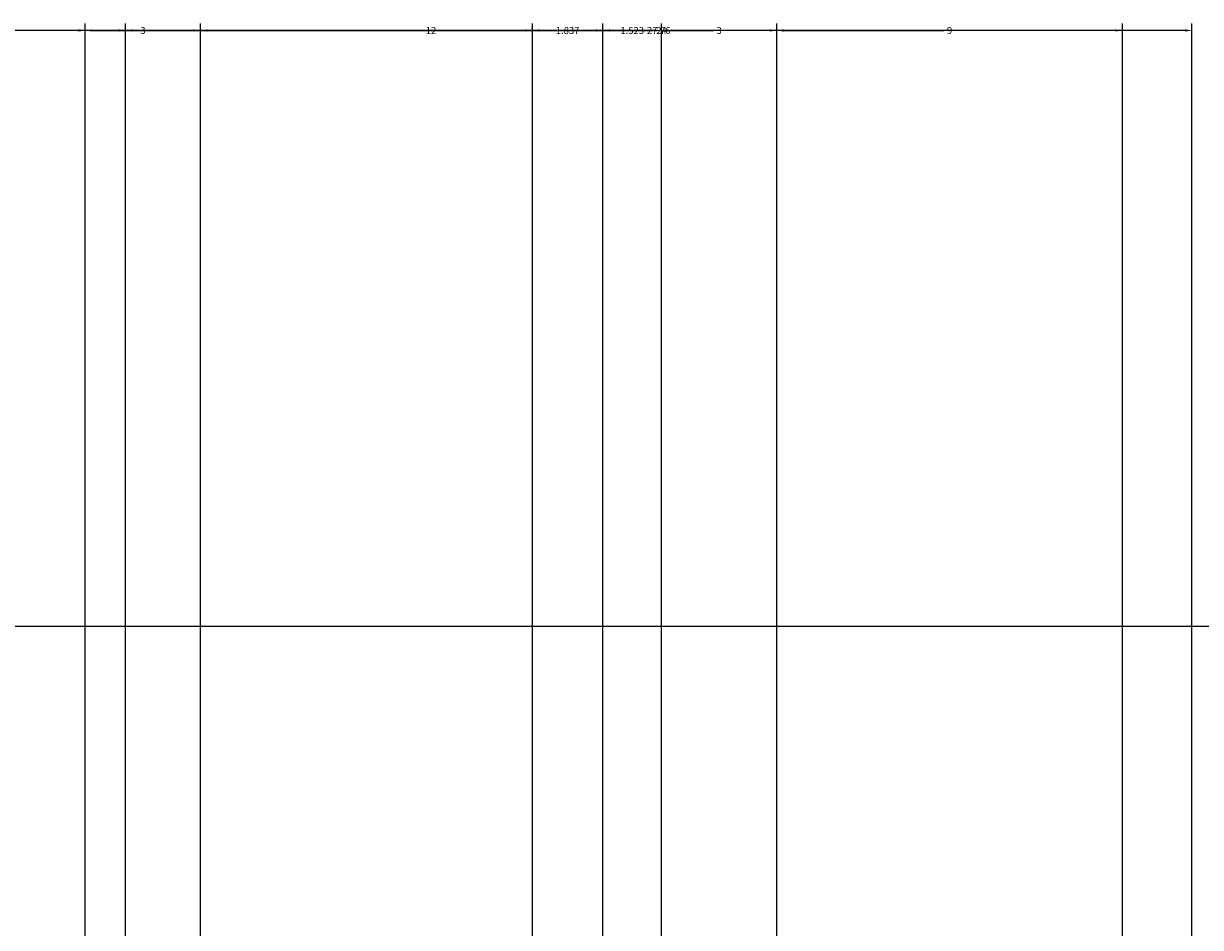
# Model space of a CAD drawing. Units: inches. Extents: x -6 to 289, y -8 to 323.
# Tile 106 of 107: x 243 to 273, y 299 to 323. Entities that reach past the tile are written whole.
import ezdxf

# ---------------------------------------------------------------- set-up
doc = ezdxf.new("R2010")
doc.units = ezdxf.units.IN
doc.header["$MEASUREMENT"] = 0
doc.layers.add('A-ANNO-DIMS', color=2, linetype='Continuous', lineweight=18)
doc.styles.get("Standard").update_dxf_attribs({"font": 'arial.ttf'})
doc.dimstyles.get("Standard").update_dxf_attribs({"dimtxt": 0.18, "dimasz": 0.18, "dimexe": 0.18, "dimexo": 0.0625, "dimgap": 0.09, "dimtad": 0, "dimtih": 1, "dimtoh": 1, "dimdec": 4, "dimzin": 0, "dimdsep": 46, "dimtxsty": 'Standard', "dimcen": 0.09, "dimadec": 0, "dimazin": 0, "dimtfac": 1, "dimtdec": 4, "dimtofl": 0, "dimtmove": 0, "dimatfit": 3, "dimfxl": 1, "dimtolj": 1, "dimtzin": 0, "dimarcsym": 0})

# ---------------------------------------------------------------- blocks, each defined once
blk = doc.blocks.new('*D14')
at = {"layer": 'A-ANNO-DIMS', "color": 0, "lineweight": -2, "transparency": 16777216}
for p, q in [((236.292, 226.951), (236.292, 322.969)), ((247.164, 162.411), (247.164, 322.969)), ((236.472, 322.789), (241.274, 322.789)), ((246.984, 322.789), (242.182, 322.789))]:
    blk.add_line(p, q, dxfattribs=at)
at = {"layer": 'A-ANNO-DIMS', "color": 0, "transparency": 16777216}
for points in [[(236.472, 322.819), (236.472, 322.759), (236.292, 322.789)], [(246.984, 322.819), (246.984, 322.759), (247.164, 322.789)]]:
    blk.add_solid(points, dxfattribs=at)
at = {"layer": 'Defpoints', "color": 0, "transparency": 16777216}
for p in [(247.164, 322.789), (236.292, 226.889), (247.164, 162.348)]:
    blk.add_point(p, dxfattribs=at)
at = {"layer": 'A-ANNO-DIMS', "color": 0, "transparency": 16777216, "insert": (241.728, 322.789), "char_height": 0.18, "attachment_point": 5}
blk.add_mtext('\\A1;10.872', dxfattribs=at)
blk = doc.blocks.new('*D15')
at = {"layer": 'A-ANNO-DIMS', "color": 0, "lineweight": -2, "transparency": 16777216}
for p, q in [((247.164, 162.411), (247.164, 322.969)), ((271.164, 7.351), (271.164, 322.969)), ((247.344, 322.789), (258.944, 322.789)), ((270.984, 322.789), (259.384, 322.789))]:
    blk.add_line(p, q, dxfattribs=at)
at = {"layer": 'A-ANNO-DIMS', "color": 0, "transparency": 16777216}
for points in [[(247.344, 322.819), (247.344, 322.759), (247.164, 322.789)], [(270.984, 322.819), (270.984, 322.759), (271.164, 322.789)]]:
    blk.add_solid(points, dxfattribs=at)
at = {"layer": 'Defpoints', "color": 0, "transparency": 16777216}
for p in [(271.164, 322.789), (247.164, 162.348), (271.164, 7.289)]:
    blk.add_point(p, dxfattribs=at)
at = {"layer": 'A-ANNO-DIMS', "color": 0, "transparency": 16777216, "insert": (259.164, 322.789), "char_height": 0.18, "attachment_point": 5}
blk.add_mtext('\\A1;24', dxfattribs=at)
blk = doc.blocks.new('*D27')
at = {"layer": 'A-ANNO-DIMS', "color": 0, "lineweight": -2, "transparency": 16777216}
for p, q in [((19.226, 307.289), (288.653, 307.289)), ((288.473, 307.109), (288.473, 277.471)), ((288.473, 247.469), (288.473, 277.107)), ((247.226, 247.289), (288.653, 247.289))]:
    blk.add_line(p, q, dxfattribs=at)
at = {"layer": 'A-ANNO-DIMS', "color": 0, "transparency": 16777216}
for points in [[(288.443, 307.109), (288.503, 307.109), (288.473, 307.289)], [(288.443, 247.469), (288.503, 247.469), (288.473, 247.289)]]:
    blk.add_solid(points, dxfattribs=at)
at = {"layer": 'Defpoints', "color": 0, "transparency": 16777216}
for p in [(19.164, 307.289), (288.473, 307.289), (247.164, 247.289)]:
    blk.add_point(p, dxfattribs=at)
at = {"layer": 'A-ANNO-DIMS', "color": 0, "transparency": 16777216, "insert": (288.473, 277.289), "char_height": 0.18, "attachment_point": 5}
blk.add_mtext('\\A1;60', dxfattribs=at)
blk = doc.blocks.new('*D81')
at = {"layer": 'A-ANNO-DIMS', "color": 0, "lineweight": -2, "transparency": 16777216}
for p, q in [((230.292, 68.842), (230.292, 322.969)), ((245.215, 66.286), (245.215, 322.969)), ((230.472, 322.789), (237.298, 322.789)), ((245.035, 322.789), (238.208, 322.789))]:
    blk.add_line(p, q, dxfattribs=at)
at = {"layer": 'A-ANNO-DIMS', "color": 0, "transparency": 16777216}
for points in [[(230.472, 322.819), (230.472, 322.759), (230.292, 322.789)], [(245.035, 322.819), (245.035, 322.759), (245.215, 322.789)]]:
    blk.add_solid(points, dxfattribs=at)
at = {"layer": 'Defpoints', "color": 0, "transparency": 16777216}
for p in [(245.215, 322.789), (230.292, 68.779), (245.215, 66.224)]:
    blk.add_point(p, dxfattribs=at)
at = {"layer": 'A-ANNO-DIMS', "color": 0, "transparency": 16777216, "insert": (237.753, 322.789), "char_height": 0.18, "attachment_point": 5}
blk.add_mtext('\\A1;14.923', dxfattribs=at)
blk = doc.blocks.new('*D82')
at = {"layer": 'A-ANNO-DIMS', "color": 0, "lineweight": -2, "transparency": 16777216}
for p, q in [((245.215, 66.286), (245.215, 322.969)), ((272.973, 66.286), (272.973, 322.969)), ((245.395, 322.789), (258.699, 322.789)), ((272.793, 322.789), (259.489, 322.789))]:
    blk.add_line(p, q, dxfattribs=at)
at = {"layer": 'A-ANNO-DIMS', "color": 0, "transparency": 16777216}
for points in [[(245.395, 322.819), (245.395, 322.759), (245.215, 322.789)], [(272.793, 322.819), (272.793, 322.759), (272.973, 322.789)]]:
    blk.add_solid(points, dxfattribs=at)
at = {"layer": 'Defpoints', "color": 0, "transparency": 16777216}
for p in [(272.973, 322.789), (245.215, 66.224), (272.973, 66.224)]:
    blk.add_point(p, dxfattribs=at)
at = {"layer": 'A-ANNO-DIMS', "color": 0, "transparency": 16777216, "insert": (259.094, 322.789), "char_height": 0.18, "attachment_point": 5}
blk.add_mtext('\\A1;27.76', dxfattribs=at)
blk = doc.blocks.new('*D98')
at = {"layer": 'A-ANNO-DIMS', "color": 0, "lineweight": -2, "transparency": 16777216}
for p, q in [((202.741, 159.411), (202.741, 322.969)), ((244.164, 159.411), (244.164, 322.969)), ((202.921, 322.789), (223.056, 322.789)), ((243.984, 322.789), (223.849, 322.789))]:
    blk.add_line(p, q, dxfattribs=at)
at = {"layer": 'A-ANNO-DIMS', "color": 0, "transparency": 16777216}
for points in [[(202.921, 322.819), (202.921, 322.759), (202.741, 322.789)], [(243.984, 322.819), (243.984, 322.759), (244.164, 322.789)]]:
    blk.add_solid(points, dxfattribs=at)
at = {"layer": 'Defpoints', "color": 0, "transparency": 16777216}
for p in [(244.164, 322.789), (202.741, 159.348), (244.164, 159.348)]:
    blk.add_point(p, dxfattribs=at)
at = {"layer": 'A-ANNO-DIMS', "color": 0, "transparency": 16777216, "insert": (223.452, 322.789), "char_height": 0.18, "attachment_point": 5}
blk.add_mtext('\\A1;41.42', dxfattribs=at)
blk = doc.blocks.new('*D99')
at = {"layer": 'A-ANNO-DIMS', "color": 0, "lineweight": -2, "transparency": 16777216}
for p, q in [((244.164, 159.411), (244.164, 322.969)), ((247.164, 162.411), (247.164, 322.969)), ((244.344, 322.789), (245.515, 322.789)), ((246.984, 322.789), (245.813, 322.789))]:
    blk.add_line(p, q, dxfattribs=at)
at = {"layer": 'A-ANNO-DIMS', "color": 0, "transparency": 16777216}
for points in [[(244.344, 322.819), (244.344, 322.759), (244.164, 322.789)], [(246.984, 322.819), (246.984, 322.759), (247.164, 322.789)]]:
    blk.add_solid(points, dxfattribs=at)
at = {"layer": 'Defpoints', "color": 0, "transparency": 16777216}
for p in [(247.164, 322.789), (247.164, 162.348), (244.164, 159.348)]:
    blk.add_point(p, dxfattribs=at)
at = {"layer": 'A-ANNO-DIMS', "color": 0, "transparency": 16777216, "insert": (245.664, 322.789), "char_height": 0.18, "attachment_point": 5}
blk.add_mtext('\\A1;3', dxfattribs=at)
blk = doc.blocks.new('*D100')
at = {"layer": 'A-ANNO-DIMS', "color": 0, "lineweight": -2, "transparency": 16777216}
for p, q in [((247.164, 162.411), (247.164, 322.969)), ((259.164, 139.351), (259.164, 322.969)), ((247.344, 322.789), (252.954, 322.789)), ((258.984, 322.789), (253.373, 322.789))]:
    blk.add_line(p, q, dxfattribs=at)
at = {"layer": 'A-ANNO-DIMS', "color": 0, "transparency": 16777216}
for points in [[(247.344, 322.819), (247.344, 322.759), (247.164, 322.789)], [(258.984, 322.819), (258.984, 322.759), (259.164, 322.789)]]:
    blk.add_solid(points, dxfattribs=at)
at = {"layer": 'Defpoints', "color": 0, "transparency": 16777216}
for p in [(259.164, 322.789), (247.164, 162.348), (259.164, 139.289)]:
    blk.add_point(p, dxfattribs=at)
at = {"layer": 'A-ANNO-DIMS', "color": 0, "transparency": 16777216, "insert": (253.164, 322.789), "char_height": 0.18, "attachment_point": 5}
blk.add_mtext('\\A1;12', dxfattribs=at)
blk = doc.blocks.new('*D108')
at = {"layer": 'A-ANNO-DIMS', "color": 0, "lineweight": -2, "transparency": 16777216}
for p, q in [((186.984, 291.541), (186.984, 322.969)), ((255.804, 291.541), (255.804, 322.969)), ((187.164, 322.789), (221, 322.789)), ((255.624, 322.789), (221.787, 322.789))]:
    blk.add_line(p, q, dxfattribs=at)
at = {"layer": 'A-ANNO-DIMS', "color": 0, "transparency": 16777216}
for points in [[(187.164, 322.819), (187.164, 322.759), (186.984, 322.789)], [(255.624, 322.819), (255.624, 322.759), (255.804, 322.789)]]:
    blk.add_solid(points, dxfattribs=at)
at = {"layer": 'Defpoints', "color": 0, "transparency": 16777216}
for p in [(255.804, 322.789), (186.984, 291.478), (255.804, 291.478)]:
    blk.add_point(p, dxfattribs=at)
at = {"layer": 'A-ANNO-DIMS', "color": 0, "transparency": 16777216, "insert": (221.394, 322.789), "char_height": 0.18, "attachment_point": 5}
blk.add_mtext('\\A1;68.82', dxfattribs=at)
blk = doc.blocks.new('*D109')
at = {"layer": 'A-ANNO-DIMS', "color": 0, "lineweight": -2, "transparency": 16777216}
for p, q in [((255.804, 291.541), (255.804, 322.969)), ((257.641, 293.728), (257.641, 322.969)), ((255.984, 322.789), (256.337, 322.789)), ((257.461, 322.789), (257.107, 322.789))]:
    blk.add_line(p, q, dxfattribs=at)
at = {"layer": 'A-ANNO-DIMS', "color": 0, "transparency": 16777216}
for points in [[(255.984, 322.819), (255.984, 322.759), (255.804, 322.789)], [(257.461, 322.819), (257.461, 322.759), (257.641, 322.789)]]:
    blk.add_solid(points, dxfattribs=at)
at = {"layer": 'Defpoints', "color": 0, "transparency": 16777216}
for p in [(257.641, 322.789), (257.641, 293.666), (255.804, 291.478)]:
    blk.add_point(p, dxfattribs=at)
at = {"layer": 'A-ANNO-DIMS', "color": 0, "transparency": 16777216, "insert": (256.722, 322.789), "char_height": 0.18, "attachment_point": 5}
blk.add_mtext('\\A1;1.837', dxfattribs=at)
blk = doc.blocks.new('*D110')
at = {"layer": 'A-ANNO-DIMS', "color": 0, "lineweight": -2, "transparency": 16777216}
for p, q in [((257.641, 293.728), (257.641, 322.969)), ((259.164, 277.105), (259.164, 322.969)), ((257.821, 322.789), (258.017, 322.789)), ((258.984, 322.789), (258.787, 322.789))]:
    blk.add_line(p, q, dxfattribs=at)
at = {"layer": 'A-ANNO-DIMS', "color": 0, "transparency": 16777216}
for points in [[(257.821, 322.819), (257.821, 322.759), (257.641, 322.789)], [(258.984, 322.819), (258.984, 322.759), (259.164, 322.789)]]:
    blk.add_solid(points, dxfattribs=at)
at = {"layer": 'Defpoints', "color": 0, "transparency": 16777216}
for p in [(259.164, 322.789), (257.641, 293.666), (259.164, 277.043)]:
    blk.add_point(p, dxfattribs=at)
at = {"layer": 'A-ANNO-DIMS', "color": 0, "transparency": 16777216, "insert": (258.402, 322.789), "char_height": 0.18, "attachment_point": 5}
blk.add_mtext('\\A1;1.523', dxfattribs=at)
blk = doc.blocks.new('*D111')
at = {"layer": 'A-ANNO-DIMS', "color": 0, "lineweight": -2, "transparency": 16777216}
for p, q in [((259.164, 277.105), (259.164, 322.969)), ((262.164, 280.105), (262.164, 322.969)), ((259.344, 322.789), (260.515, 322.789)), ((261.984, 322.789), (260.813, 322.789))]:
    blk.add_line(p, q, dxfattribs=at)
at = {"layer": 'A-ANNO-DIMS', "color": 0, "transparency": 16777216}
for points in [[(259.344, 322.819), (259.344, 322.759), (259.164, 322.789)], [(261.984, 322.819), (261.984, 322.759), (262.164, 322.789)]]:
    blk.add_solid(points, dxfattribs=at)
at = {"layer": 'Defpoints', "color": 0, "transparency": 16777216}
for p in [(262.164, 322.789), (262.164, 280.043), (259.164, 277.043)]:
    blk.add_point(p, dxfattribs=at)
at = {"layer": 'A-ANNO-DIMS', "color": 0, "transparency": 16777216, "insert": (260.664, 322.789), "char_height": 0.18, "attachment_point": 5}
blk.add_mtext('\\A1;3', dxfattribs=at)
blk = doc.blocks.new('*D112')
at = {"layer": 'A-ANNO-DIMS', "color": 0, "lineweight": -2, "transparency": 16777216}
for p, q in [((262.164, 280.105), (262.164, 322.969)), ((271.164, 259.351), (271.164, 322.969)), ((262.344, 322.789), (266.515, 322.789)), ((270.984, 322.789), (266.813, 322.789))]:
    blk.add_line(p, q, dxfattribs=at)
at = {"layer": 'A-ANNO-DIMS', "color": 0, "transparency": 16777216}
for points in [[(262.344, 322.819), (262.344, 322.759), (262.164, 322.789)], [(270.984, 322.819), (270.984, 322.759), (271.164, 322.789)]]:
    blk.add_solid(points, dxfattribs=at)
at = {"layer": 'Defpoints', "color": 0, "transparency": 16777216}
for p in [(271.164, 322.789), (262.164, 280.043), (271.164, 259.289)]:
    blk.add_point(p, dxfattribs=at)
at = {"layer": 'A-ANNO-DIMS', "color": 0, "transparency": 16777216, "insert": (266.664, 322.789), "char_height": 0.18, "attachment_point": 5}
blk.add_mtext('\\A1;9', dxfattribs=at)
blk = doc.blocks.new('*D118')
at = {"layer": 'A-ANNO-DIMS', "color": 0, "lineweight": -2, "transparency": 16777216}
for p, q in [((118.226, 307.289), (288.653, 307.289)), ((288.473, 307.109), (288.473, 300.659)), ((288.473, 293.846), (288.473, 300.295)), ((257.703, 293.666), (288.653, 293.666))]:
    blk.add_line(p, q, dxfattribs=at)
at = {"layer": 'A-ANNO-DIMS', "color": 0, "transparency": 16777216}
for points in [[(288.443, 307.109), (288.503, 307.109), (288.473, 307.289)], [(288.443, 293.846), (288.503, 293.846), (288.473, 293.666)]]:
    blk.add_solid(points, dxfattribs=at)
at = {"layer": 'Defpoints', "color": 0, "transparency": 16777216}
for p in [(118.164, 307.289), (288.473, 307.289), (257.641, 293.666)]:
    blk.add_point(p, dxfattribs=at)
at = {"layer": 'A-ANNO-DIMS', "color": 0, "transparency": 16777216, "insert": (288.473, 300.477), "char_height": 0.18, "attachment_point": 5}
blk.add_mtext('\\A1;13.623', dxfattribs=at)

msp = doc.modelspace()

# ---------------------------------------------------------------- dimensions: what is measured, and where the dimension line sits
at = {"layer": 'A-ANNO-DIMS'}
for base, p1, p2, override, picture, middle in [((255.8036, 322.7888), (186.9837, 291.4781), (255.8036, 291.4781), {"dimdec": 2, "dimlfac": 1, "dimrnd": 0, "dimzin": 0, "dimdsep": 46, "dimlunit": 2}, '*D108', (221.3936, 322.7888)), ((244.1638, 322.7888), (202.741, 159.3484), (244.1638, 159.3484), {"dimdec": 2, "dimlfac": 1, "dimrnd": 0, "dimzin": 0, "dimdsep": 46, "dimlunit": 2}, '*D98', (223.4524, 322.7888)), ((245.2146, 322.7888), (230.2918, 68.7795), (245.2146, 66.2238), {"dimdec": 3, "dimlfac": 1, "dimrnd": 0, "dimzin": 0, "dimdsep": 46, "dimlunit": 2}, '*D81', (237.7532, 322.7888)), ((247.1638, 322.7888), (236.2918, 226.8887), (247.1638, 162.3484), {"dimdec": 3, "dimlfac": 1, "dimrnd": 0, "dimzin": 0, "dimdsep": 46, "dimlunit": 2}, '*D14', (241.7278, 322.7888)), ((247.1638, 322.7888), (244.1638, 159.3484), (247.1638, 162.3484), {"dimdec": 0, "dimlfac": 1, "dimrnd": 0, "dimzin": 0, "dimdsep": 46, "dimlunit": 2}, '*D99', (245.6638, 322.7888)), ((272.9733, 322.7888), (245.2146, 66.2238), (272.9733, 66.2238), {"dimdec": 2, "dimlfac": 1, "dimrnd": 0, "dimzin": 0, "dimdsep": 46, "dimlunit": 2}, '*D82', (259.0939, 322.7888)), ((271.1638, 322.7888), (247.1638, 162.3484), (271.1638, 7.2888), {"dimdec": 0, "dimlfac": 1, "dimrnd": 0, "dimzin": 0, "dimdsep": 46, "dimlunit": 2}, '*D15', (259.1638, 322.7888)), ((259.1638, 322.7888), (247.1638, 162.3484), (259.1638, 139.2888), {"dimdec": 0, "dimlfac": 1, "dimrnd": 0, "dimzin": 0, "dimdsep": 46, "dimlunit": 2}, '*D100', (253.1638, 322.7888)), ((257.6407, 322.7888), (255.8036, 291.4781), (257.6407, 293.6657), {"dimdec": 3, "dimlfac": 1, "dimrnd": 0, "dimzin": 0, "dimdsep": 46, "dimlunit": 2}, '*D109', (256.7221, 322.7888)), ((259.1638, 322.7888), (257.6407, 293.6657), (259.1638, 277.0427), {"dimdec": 3, "dimlfac": 1, "dimrnd": 0, "dimzin": 0, "dimdsep": 46, "dimlunit": 2}, '*D110', (258.4022, 322.7888)), ((262.1638, 322.7888), (259.1638, 277.0427), (262.1638, 280.0427), {"dimdec": 0, "dimlfac": 1, "dimrnd": 0, "dimzin": 0, "dimdsep": 46, "dimlunit": 2}, '*D111', (260.6638, 322.7888)), ((271.1638, 322.7888), (262.1638, 280.0427), (271.1638, 259.2888), {"dimdec": 0, "dimlfac": 1, "dimrnd": 0, "dimzin": 0, "dimdsep": 46, "dimlunit": 2}, '*D112', (266.6638, 322.7888))]:
    dim = msp.add_linear_dim(base=base, p1=p1, p2=p2, dimstyle='Standard', override=override, dxfattribs=at)
    dim.commit()
    dim.dimension.update_dxf_attribs({"geometry": picture, "text_midpoint": middle})
for p1, p2, override, picture, middle in [((247.1638, 247.2888), (19.1638, 307.2888), {"dimdec": 0, "dimlfac": 1, "dimrnd": 0, "dimzin": 0, "dimdsep": 46, "dimlunit": 2}, '*D27', (288.4733, 277.2888)), ((257.6407, 293.6657), (118.1638, 307.2888), {"dimdec": 3, "dimlfac": 1, "dimrnd": 0, "dimzin": 0, "dimdsep": 46, "dimlunit": 2}, '*D118', (288.4733, 300.4773))]:
    dim = msp.add_linear_dim(base=(288.4733, 307.2888), p1=p1, p2=p2, angle=90, dimstyle='Standard', override=override, dxfattribs=at)
    dim.commit()
    dim.dimension.update_dxf_attribs({"geometry": picture, "text_midpoint": middle})

doc.saveas('drawing.dxf')
